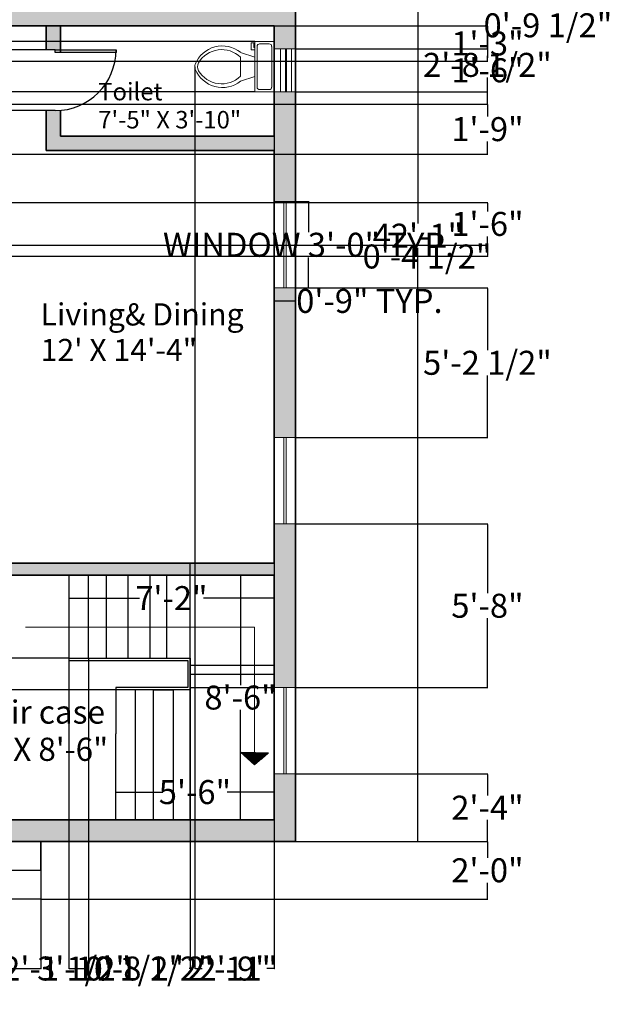
# Model space of a CAD drawing. Units: inches. Extents: x 46 to 946, y 121 to 740.
# Tile 3 of 4: x 287 to 533, y 121 to 531. Entities that reach past the tile are written whole.
import ezdxf

# ---------------------------------------------------------------- set-up
doc = ezdxf.new("R2010")
doc.units = ezdxf.units.IN
doc.header["$MEASUREMENT"] = 0
for name, color, linetype, lineweight in [('A-ANNO-DIMS', 2, 'Continuous', 18), ('A-ANNO-SYMB', 7, 'Continuous', 18), ('A-AREA-IDEN', 7, 'Continuous', 25), ('A-DOOR', 3, 'Continuous', 25), ('A-FLOR-FIXT', 9, 'Continuous', 18), ('A-FLOR-STRS', 7, 'Continuous', 25), ('A-GLAZ', 4, 'Continuous', 18), ('A-WALL', 7, 'Continuous', 35), ('A-WALL-PATT', 8, 'Continuous', 13)]:
    doc.layers.add(name, color=color, linetype=linetype, lineweight=lineweight)
doc.styles.get("Standard").update_dxf_attribs({"font": 'arial.ttf'})
doc.dimstyles.get("Standard").update_dxf_attribs({"dimtxt": 10, "dimasz": 0.18, "dimexe": 0.18, "dimexo": 0.0625, "dimgap": 0.09, "dimtad": 0, "dimtih": 1, "dimtoh": 1, "dimdec": 0, "dimzin": 0, "dimdsep": 46, "dimlunit": 3, "dimtxsty": 'Standard', "dimcen": 0.09, "dimadec": 0, "dimazin": 0, "dimtfac": 1, "dimtdec": 0, "dimtofl": 0, "dimtmove": 0, "dimatfit": 3, "dimfxl": 1, "dimtolj": 1, "dimtzin": 0, "dimarcsym": 0})

# ---------------------------------------------------------------- blocks, each defined once
blk = doc.blocks.new('*U3')
for p, q in [((0, 0), (0, -6)), ((40, 0), (40, -6))]:
    blk.add_line(p, q)
blk.add_lwpolyline([(0, 0), (0, 40), (1.75, 40), (1.75, 0)], close=True)
blk.add_arc((0, 0), 40, 0, 90)
blk = doc.blocks.new('*D7')
at = {"layer": 'A-ANNO-DIMS', "color": 0, "lineweight": -2, "transparency": 16777216}
for p, q in [((307.86, 291.97), (307.86, 289.72)), ((393.48, 291.97), (393.48, 289.72)), ((308.04, 289.9), (337.33, 289.9)), ((393.3, 289.9), (364.01, 289.9))]:
    blk.add_line(p, q, dxfattribs=at)
at = {"layer": 'A-ANNO-DIMS', "color": 0, "transparency": 16777216}
for points in [[(308.04, 289.93), (308.04, 289.87), (307.86, 289.9)], [(393.3, 289.93), (393.3, 289.87), (393.48, 289.9)]]:
    blk.add_solid(points, dxfattribs=at)
at = {"layer": 'Defpoints', "color": 0, "transparency": 16777216}
for p in [(307.86, 292.03), (393.48, 292.03), (393.48, 289.9)]:
    blk.add_point(p, dxfattribs=at)
at = {"layer": 'A-ANNO-DIMS', "color": 0, "transparency": 16777216, "insert": (350.67, 289.9), "char_height": 10, "attachment_point": 5}
blk.add_mtext('\\A1;7\'-2"', dxfattribs=at)
blk = doc.blocks.new('*D8')
at = {"layer": 'A-ANNO-DIMS', "color": 0, "lineweight": -2, "transparency": 16777216}
for p, q in [((387.34, 299.46), (379.31, 299.46)), ((379.49, 299.28), (379.49, 253.66)), ((379.49, 197.64), (379.49, 243.27)), ((387.34, 197.46), (379.31, 197.46))]:
    blk.add_line(p, q, dxfattribs=at)
at = {"layer": 'A-ANNO-DIMS', "color": 0, "transparency": 16777216}
for points in [[(379.46, 299.28), (379.52, 299.28), (379.49, 299.46)], [(379.46, 197.64), (379.52, 197.64), (379.49, 197.46)]]:
    blk.add_solid(points, dxfattribs=at)
at = {"layer": 'Defpoints', "color": 0, "transparency": 16777216}
for p in [(387.4, 299.46), (379.49, 197.46), (387.4, 197.46)]:
    blk.add_point(p, dxfattribs=at)
at = {"layer": 'A-ANNO-DIMS', "color": 0, "transparency": 16777216, "insert": (379.49, 248.46), "char_height": 10, "attachment_point": 5}
blk.add_mtext('\\A1;8\'-6"', dxfattribs=at)
blk = doc.blocks.new('*D9')
at = {"layer": 'A-ANNO-DIMS', "color": 0, "lineweight": -2, "transparency": 16777216}
for p, q in [((327.48, 197.52), (327.48, 209.23)), ((327.66, 209.05), (347.1, 209.05)), ((393.3, 209.05), (373.86, 209.05)), ((393.48, 197.52), (393.48, 209.23))]:
    blk.add_line(p, q, dxfattribs=at)
at = {"layer": 'A-ANNO-DIMS', "color": 0, "transparency": 16777216}
for points in [[(327.66, 209.08), (327.66, 209.02), (327.48, 209.05)], [(393.3, 209.08), (393.3, 209.02), (393.48, 209.05)]]:
    blk.add_solid(points, dxfattribs=at)
at = {"layer": 'Defpoints', "color": 0, "transparency": 16777216}
for p in [(393.48, 209.05), (327.48, 197.46), (393.48, 197.46)]:
    blk.add_point(p, dxfattribs=at)
at = {"layer": 'A-ANNO-DIMS', "color": 0, "transparency": 16777216, "insert": (360.48, 209.05), "char_height": 10, "attachment_point": 5}
blk.add_mtext('\\A1;5\'-6"', dxfattribs=at)
blk = doc.blocks.new('*D11')
at = {"layer": 'A-ANNO-DIMS', "color": 0, "lineweight": -2, "transparency": 16777216}
for p, q in [((402.54, 693.46), (453.64, 693.46)), ((453.46, 693.28), (453.46, 446.07)), ((453.46, 188.64), (453.46, 435.85)), ((402.54, 188.46), (453.64, 188.46))]:
    blk.add_line(p, q, dxfattribs=at)
at = {"layer": 'A-ANNO-DIMS', "color": 0, "transparency": 16777216}
for points in [[(453.43, 693.28), (453.49, 693.28), (453.46, 693.46)], [(453.43, 188.64), (453.49, 188.64), (453.46, 188.46)]]:
    blk.add_solid(points, dxfattribs=at)
at = {"layer": 'Defpoints', "color": 0, "transparency": 16777216}
for p in [(402.48, 693.46), (402.48, 188.46), (453.46, 188.46)]:
    blk.add_point(p, dxfattribs=at)
at = {"layer": 'A-ANNO-DIMS', "color": 0, "transparency": 16777216, "insert": (453.46, 440.96), "char_height": 10, "attachment_point": 5}
blk.add_mtext('\\A1;42\'-1"', dxfattribs=at)
blk = doc.blocks.new('*U13')
for p, q in [((241, -152), (241, -51)), ((-203, -216), (-203, -203)), ((-178, -203), (-178, -241)), ((-102, -203), (-152, -356)), ((102, -203), (152, -356)), ((-254, -216), (-203, -216)), ((-254, -241), (-254, -216)), ((-178, -241), (-254, -241)), ((102, -356), (-102, -356))]:
    blk.add_line(p, q)
blk.add_lwpolyline([(267, -203), (267, 0), (-267, 0), (-267, -203)], close=True)
for points in [[(-241, -51), (-241, -152)], [(216, -25), (-216, -25)], [(-216, -178), (216, -178)]]:
    blk.add_lwpolyline(points)
for centre, radius, start, end in [((-219, -48), 22.5, 81.8699, 188.1301), ((219, -48), 22.5, 351.8699, 98.1301), ((-219, -156), 22.5, 171.8699, 278.1301), ((219, -156), 22.5, 261.8699, 8.1301), ((89, -548), 309, 141.4691, 247.9714), ((107, -554), 288, 136.3677, 238.9468), ((-89, -548), 309, 292.0284, 38.5307), ((-107, -554), 288, 301.053, 43.6321), ((0, -708), 102, 245.7318, 294.2682), ((0, -737), 102, 254.8605, 285.1395)]:
    blk.add_arc(centre, radius, start, end)
blk = doc.blocks.new('WIN-36IN')
for p, q in [((9, 36), (0, 36)), ((0, 0), (0, 36)), ((4, 36), (4, 0)), ((5, 36), (5, 0)), ((9, 36), (9, 0)), ((9, 0), (0, 0)), ((9, 0), (0, 0))]:
    blk.add_line(p, q)
blk = doc.blocks.new('ARROW-DIRECTION')
h = blk.add_hatch()
h.set_pattern_fill('ANSI31', color=256, angle=180)
h.set_pattern_definition([(225, (391.19844, 225.63338), (0.088388348, -0.088388348), [])])
h.paths.add_polyline_path([(0, 0.27), (11.71, 0), (5.84, 5.18)])
for p, q in [((5.84, 5.18), (0, 0.27)), ((5.84, 5.18), (11.71, 0)), ((11.71, 0), (5.84, 5.18))]:
    blk.add_line(p, q)
blk = doc.blocks.new('*D20')
at = {"layer": 'A-ANNO-DIMS', "color": 0, "lineweight": -2, "transparency": 16777216}
for p, q in [((402.54, 455.17), (408.06, 455.17)), ((407.88, 454.99), (407.88, 442.43)), ((407.88, 419.35), (407.88, 431.9)), ((402.54, 419.17), (408.06, 419.17))]:
    blk.add_line(p, q, dxfattribs=at)
at = {"layer": 'A-ANNO-DIMS', "color": 0, "transparency": 16777216}
for points in [[(407.85, 454.99), (407.91, 454.99), (407.88, 455.17)], [(407.85, 419.35), (407.91, 419.35), (407.88, 419.17)]]:
    blk.add_solid(points, dxfattribs=at)
at = {"layer": 'Defpoints', "color": 0, "transparency": 16777216}
for p in [(402.48, 455.17), (407.88, 455.17), (402.48, 419.17)]:
    blk.add_point(p, dxfattribs=at)
at = {"layer": 'A-ANNO-DIMS', "color": 0, "transparency": 16777216, "insert": (407.88, 437.17), "char_height": 10, "attachment_point": 5}
blk.add_mtext('\\A1;WINDOW 3\'-0" TYP.', dxfattribs=at)
blk = doc.blocks.new('*D21')
at = {"layer": 'A-ANNO-DIMS', "color": 0, "lineweight": -2, "transparency": 16777216}
for p, q in [((393.48, 419.1), (393.48, 413.59)), ((402.48, 419.1), (402.48, 413.59)), ((393.66, 413.77), (402.3, 413.77)), ((402.48, 413.77), (402.66, 413.77))]:
    blk.add_line(p, q, dxfattribs=at)
at = {"layer": 'A-ANNO-DIMS', "color": 0, "transparency": 16777216}
for points in [[(393.66, 413.8), (393.66, 413.74), (393.48, 413.77)], [(402.3, 413.8), (402.3, 413.74), (402.48, 413.77)]]:
    blk.add_solid(points, dxfattribs=at)
at = {"layer": 'Defpoints', "color": 0, "transparency": 16777216}
for p in [(393.48, 419.17), (402.48, 419.17), (402.48, 413.77)]:
    blk.add_point(p, dxfattribs=at)
at = {"layer": 'A-ANNO-DIMS', "color": 0, "transparency": 16777216, "insert": (433.22, 413.77), "char_height": 10, "attachment_point": 5}
blk.add_mtext('\\A1;0\'-9" TYP.', dxfattribs=at)
blk = doc.blocks.new('*D25')
at = {"layer": 'A-ANNO-DIMS', "color": 0, "lineweight": -2, "transparency": 16777216}
for p, q in [((249.48, 164.4), (249.48, 135.33)), ((296.21, 164.4), (296.21, 135.33)), ((249.66, 135.51), (296.03, 135.51)), ((296.21, 135.51), (296.39, 135.51))]:
    blk.add_line(p, q, dxfattribs=at)
at = {"layer": 'A-ANNO-DIMS', "color": 0, "transparency": 16777216}
for points in [[(249.66, 135.54), (249.66, 135.48), (249.48, 135.51)], [(296.03, 135.54), (296.03, 135.48), (296.21, 135.51)]]:
    blk.add_solid(points, dxfattribs=at)
at = {"layer": 'Defpoints', "color": 0, "transparency": 16777216}
for p in [(249.48, 164.46), (296.21, 164.46), (296.21, 135.51)]:
    blk.add_point(p, dxfattribs=at)
at = {"layer": 'A-ANNO-DIMS', "color": 0, "transparency": 16777216, "insert": (325.3, 135.51), "char_height": 10, "attachment_point": 5}
blk.add_mtext('\\A1;3\'-10 1/2"', dxfattribs=at)
blk = doc.blocks.new('*D26')
at = {"layer": 'A-ANNO-DIMS', "color": 0, "lineweight": -2, "transparency": 16777216}
for p, q in [((296.27, 188.46), (482.61, 188.46)), ((482.43, 188.28), (482.43, 181.66)), ((482.43, 164.64), (482.43, 171.27)), ((296.27, 164.46), (482.61, 164.46))]:
    blk.add_line(p, q, dxfattribs=at)
at = {"layer": 'A-ANNO-DIMS', "color": 0, "transparency": 16777216}
for points in [[(482.4, 188.28), (482.46, 188.28), (482.43, 188.46)], [(482.4, 164.64), (482.46, 164.64), (482.43, 164.46)]]:
    blk.add_solid(points, dxfattribs=at)
at = {"layer": 'Defpoints', "color": 0, "transparency": 16777216}
for p in [(296.21, 188.46), (482.43, 188.46), (296.21, 164.46)]:
    blk.add_point(p, dxfattribs=at)
at = {"layer": 'A-ANNO-DIMS', "color": 0, "transparency": 16777216, "insert": (482.43, 176.46), "char_height": 10, "attachment_point": 5}
blk.add_mtext('\\A1;2\'-0"', dxfattribs=at)
blk = doc.blocks.new('*D37')
at = {"layer": 'A-ANNO-DIMS', "color": 0, "lineweight": -2, "transparency": 16777216}
for p, q in [((402.54, 216.63), (482.61, 216.63)), ((482.43, 216.45), (482.43, 207.66)), ((482.43, 188.64), (482.43, 197.44)), ((402.54, 188.46), (482.61, 188.46))]:
    blk.add_line(p, q, dxfattribs=at)
at = {"layer": 'A-ANNO-DIMS', "color": 0, "transparency": 16777216}
for points in [[(482.4, 216.45), (482.46, 216.45), (482.43, 216.63)], [(482.4, 188.64), (482.46, 188.64), (482.43, 188.46)]]:
    blk.add_solid(points, dxfattribs=at)
at = {"layer": 'Defpoints', "color": 0, "transparency": 16777216}
for p in [(402.48, 216.63), (482.43, 216.63), (402.48, 188.46)]:
    blk.add_point(p, dxfattribs=at)
at = {"layer": 'A-ANNO-DIMS', "color": 0, "transparency": 16777216, "insert": (482.43, 202.55), "char_height": 10, "attachment_point": 5}
blk.add_mtext('\\A1;2\'-4"', dxfattribs=at)
blk = doc.blocks.new('*D38')
at = {"layer": 'A-ANNO-DIMS', "color": 0, "lineweight": -2, "transparency": 16777216}
for p, q in [((402.54, 320.8), (482.61, 320.8)), ((482.43, 320.62), (482.43, 291.91)), ((482.43, 252.81), (482.43, 281.52)), ((402.54, 252.63), (482.61, 252.63))]:
    blk.add_line(p, q, dxfattribs=at)
at = {"layer": 'A-ANNO-DIMS', "color": 0, "transparency": 16777216}
for points in [[(482.4, 320.62), (482.46, 320.62), (482.43, 320.8)], [(482.4, 252.81), (482.46, 252.81), (482.43, 252.63)]]:
    blk.add_solid(points, dxfattribs=at)
at = {"layer": 'Defpoints', "color": 0, "transparency": 16777216}
for p in [(402.48, 320.8), (482.43, 320.8), (402.48, 252.63)]:
    blk.add_point(p, dxfattribs=at)
at = {"layer": 'A-ANNO-DIMS', "color": 0, "transparency": 16777216, "insert": (482.43, 286.72), "char_height": 10, "attachment_point": 5}
blk.add_mtext('\\A1;5\'-8"', dxfattribs=at)
blk = doc.blocks.new('*D39')
at = {"layer": 'A-ANNO-DIMS', "color": 0, "lineweight": -2, "transparency": 16777216}
for p, q in [((402.54, 419.17), (482.61, 419.17)), ((482.43, 418.99), (482.43, 393.25)), ((482.43, 356.98), (482.43, 382.72)), ((402.54, 356.8), (482.61, 356.8))]:
    blk.add_line(p, q, dxfattribs=at)
at = {"layer": 'A-ANNO-DIMS', "color": 0, "transparency": 16777216}
for points in [[(482.4, 418.99), (482.46, 418.99), (482.43, 419.17)], [(482.4, 356.98), (482.46, 356.98), (482.43, 356.8)]]:
    blk.add_solid(points, dxfattribs=at)
at = {"layer": 'Defpoints', "color": 0, "transparency": 16777216}
for p in [(402.48, 419.17), (482.43, 419.17), (402.48, 356.8)]:
    blk.add_point(p, dxfattribs=at)
at = {"layer": 'A-ANNO-DIMS', "color": 0, "transparency": 16777216, "insert": (482.43, 387.98), "char_height": 10, "attachment_point": 5}
blk.add_mtext('\\A1;5\'-2 1/2"', dxfattribs=at)
blk = doc.blocks.new('*D40')
at = {"layer": 'A-ANNO-DIMS', "color": 0, "lineweight": -2, "transparency": 16777216}
for p, q in [((393.54, 528.46), (482.61, 528.46)), ((482.43, 528.46), (482.43, 528.64)), ((482.43, 528.64), (482.61, 528.64)), ((482.43, 519.05), (482.43, 528.28)), ((402.54, 518.87), (482.61, 518.87))]:
    blk.add_line(p, q, dxfattribs=at)
at = {"layer": 'A-ANNO-DIMS', "color": 0, "transparency": 16777216}
for points in [[(482.4, 528.28), (482.46, 528.28), (482.43, 528.46)], [(482.4, 519.05), (482.46, 519.05), (482.43, 518.87)]]:
    blk.add_solid(points, dxfattribs=at)
at = {"layer": 'Defpoints', "color": 0, "transparency": 16777216}
for p in [(393.48, 528.46), (482.43, 528.46), (402.48, 518.87)]:
    blk.add_point(p, dxfattribs=at)
at = {"layer": 'A-ANNO-DIMS', "color": 0, "transparency": 16777216, "insert": (507.64, 528.64), "char_height": 10, "attachment_point": 5}
blk.add_mtext('\\A1;0\'-9 1/2"', dxfattribs=at)
blk = doc.blocks.new('*D41')
at = {"layer": 'A-ANNO-DIMS', "color": 0, "lineweight": -2, "transparency": 16777216}
for p, q in [((402.54, 518.87), (482.61, 518.87)), ((482.43, 518.69), (482.43, 515.07)), ((402.54, 500.87), (482.61, 500.87)), ((482.43, 501.05), (482.43, 504.68))]:
    blk.add_line(p, q, dxfattribs=at)
at = {"layer": 'A-ANNO-DIMS', "color": 0, "transparency": 16777216}
for points in [[(482.4, 518.69), (482.46, 518.69), (482.43, 518.87)], [(482.4, 501.05), (482.46, 501.05), (482.43, 500.87)]]:
    blk.add_solid(points, dxfattribs=at)
at = {"layer": 'Defpoints', "color": 0, "transparency": 16777216}
for p in [(402.48, 518.87), (482.43, 518.87), (402.48, 500.87)]:
    blk.add_point(p, dxfattribs=at)
at = {"layer": 'A-ANNO-DIMS', "color": 0, "transparency": 16777216, "insert": (482.43, 509.87), "char_height": 10, "attachment_point": 5}
blk.add_mtext('\\A1;1\'-6"', dxfattribs=at)
blk = doc.blocks.new('*D44')
at = {"layer": 'A-ANNO-DIMS', "color": 0, "lineweight": -2, "transparency": 16777216}
for p, q in [((256.37, 188.4), (256.37, 135.33)), ((281.69, 188.4), (281.69, 135.33)), ((256.55, 135.51), (281.51, 135.51)), ((281.69, 135.51), (281.87, 135.51))]:
    blk.add_line(p, q, dxfattribs=at)
at = {"layer": 'A-ANNO-DIMS', "color": 0, "transparency": 16777216}
for points in [[(256.55, 135.54), (256.55, 135.48), (256.37, 135.51)], [(281.51, 135.54), (281.51, 135.48), (281.69, 135.51)]]:
    blk.add_solid(points, dxfattribs=at)
at = {"layer": 'Defpoints', "color": 0, "transparency": 16777216}
for p in [(256.37, 188.46), (281.69, 188.46), (281.69, 135.51)]:
    blk.add_point(p, dxfattribs=at)
at = {"layer": 'A-ANNO-DIMS', "color": 0, "transparency": 16777216, "insert": (306.99, 135.51), "char_height": 10, "attachment_point": 5}
blk.add_mtext('\\A1;2\'-1 1/2"', dxfattribs=at)
blk = doc.blocks.new('*D48')
at = {"layer": 'A-ANNO-DIMS', "color": 0, "lineweight": -2, "transparency": 16777216}
for p, q in [((188.89, 454.75), (482.61, 454.75)), ((482.43, 454.57), (482.43, 451.05)), ((482.43, 437.15), (482.43, 440.66)), ((188.89, 436.97), (482.61, 436.97))]:
    blk.add_line(p, q, dxfattribs=at)
at = {"layer": 'A-ANNO-DIMS', "color": 0, "transparency": 16777216}
for points in [[(482.4, 454.57), (482.46, 454.57), (482.43, 454.75)], [(482.4, 437.15), (482.46, 437.15), (482.43, 436.97)]]:
    blk.add_solid(points, dxfattribs=at)
at = {"layer": 'Defpoints', "color": 0, "transparency": 16777216}
for p in [(188.83, 454.75), (482.43, 454.75), (188.83, 436.97)]:
    blk.add_point(p, dxfattribs=at)
at = {"layer": 'A-ANNO-DIMS', "color": 0, "transparency": 16777216, "insert": (482.43, 445.86), "char_height": 10, "attachment_point": 5}
blk.add_mtext('\\A1;1\'-6"', dxfattribs=at)
blk = doc.blocks.new('*D50')
at = {"layer": 'A-ANNO-DIMS', "color": 0, "lineweight": -2, "transparency": 16777216}
for p, q in [((195.54, 495.84), (482.61, 495.84)), ((482.43, 495.66), (482.43, 490.57)), ((482.43, 475.08), (482.43, 480.18)), ((195.54, 474.9), (482.61, 474.9))]:
    blk.add_line(p, q, dxfattribs=at)
at = {"layer": 'A-ANNO-DIMS', "color": 0, "transparency": 16777216}
for points in [[(482.4, 495.66), (482.46, 495.66), (482.43, 495.84)], [(482.4, 475.08), (482.46, 475.08), (482.43, 474.9)]]:
    blk.add_solid(points, dxfattribs=at)
at = {"layer": 'Defpoints', "color": 0, "transparency": 16777216}
for p in [(195.48, 495.84), (482.43, 495.84), (195.48, 474.9)]:
    blk.add_point(p, dxfattribs=at)
at = {"layer": 'A-ANNO-DIMS', "color": 0, "transparency": 16777216, "insert": (482.43, 485.37), "char_height": 10, "attachment_point": 5}
blk.add_mtext('\\A1;1\'-9"', dxfattribs=at)
blk = doc.blocks.new('*D55')
at = {"layer": 'A-ANNO-DIMS', "color": 0, "lineweight": -2, "transparency": 16777216}
for p, q in [((307.8, 299.46), (85.35, 299.46)), ((85.53, 299.28), (85.53, 287.43)), ((85.53, 265.06), (85.53, 276.91)), ((307.8, 264.88), (85.35, 264.88))]:
    blk.add_line(p, q, dxfattribs=at)
at = {"layer": 'A-ANNO-DIMS', "color": 0, "transparency": 16777216}
for points in [[(85.5, 299.28), (85.56, 299.28), (85.53, 299.46)], [(85.5, 265.06), (85.56, 265.06), (85.53, 264.88)]]:
    blk.add_solid(points, dxfattribs=at)
at = {"layer": 'Defpoints', "color": 0, "transparency": 16777216}
for p in [(307.86, 299.46), (85.53, 264.88), (307.86, 264.88)]:
    blk.add_point(p, dxfattribs=at)
at = {"layer": 'A-ANNO-DIMS', "color": 0, "transparency": 16777216, "insert": (85.53, 282.17), "char_height": 10, "attachment_point": 5}
blk.add_mtext('\\A1;2\'-10 1/2"', dxfattribs=at)
blk = doc.blocks.new('*D56')
at = {"layer": 'A-ANNO-DIMS', "color": 0, "lineweight": -2, "transparency": 16777216}
for p, q in [((307.86, 264.81), (307.86, 135.33)), ((316.14, 264.81), (316.14, 135.33)), ((308.04, 135.51), (315.96, 135.51)), ((316.14, 135.51), (316.32, 135.51))]:
    blk.add_line(p, q, dxfattribs=at)
at = {"layer": 'A-ANNO-DIMS', "color": 0, "transparency": 16777216}
for points in [[(308.04, 135.54), (308.04, 135.48), (307.86, 135.51)], [(315.96, 135.54), (315.96, 135.48), (316.14, 135.51)]]:
    blk.add_solid(points, dxfattribs=at)
at = {"layer": 'Defpoints', "color": 0, "transparency": 16777216}
for p in [(307.86, 264.88), (316.14, 264.88), (316.14, 135.51)]:
    blk.add_point(p, dxfattribs=at)
at = {"layer": 'A-ANNO-DIMS', "color": 0, "transparency": 16777216, "insert": (341.35, 135.51), "char_height": 10, "attachment_point": 5}
blk.add_mtext('\\A1;0\'-8 1/2"', dxfattribs=at)
blk = doc.blocks.new('*D57')
at = {"layer": 'A-ANNO-DIMS', "color": 0, "lineweight": -2, "transparency": 16777216}
for p, q in [((327.41, 251.63), (85.35, 251.63)), ((85.53, 251.45), (85.53, 229.74)), ((85.53, 197.64), (85.53, 219.35)), ((327.41, 197.46), (85.35, 197.46))]:
    blk.add_line(p, q, dxfattribs=at)
at = {"layer": 'A-ANNO-DIMS', "color": 0, "transparency": 16777216}
for points in [[(85.5, 251.45), (85.56, 251.45), (85.53, 251.63)], [(85.5, 197.64), (85.56, 197.64), (85.53, 197.46)]]:
    blk.add_solid(points, dxfattribs=at)
at = {"layer": 'Defpoints', "color": 0, "transparency": 16777216}
for p in [(327.48, 251.63), (85.53, 197.46), (327.48, 197.46)]:
    blk.add_point(p, dxfattribs=at)
at = {"layer": 'A-ANNO-DIMS', "color": 0, "transparency": 16777216, "insert": (85.53, 224.55), "char_height": 10, "attachment_point": 5}
blk.add_mtext('\\A1;4\'-6"', dxfattribs=at)
blk = doc.blocks.new('*D58')
at = {"layer": 'A-ANNO-DIMS', "color": 0, "lineweight": -2, "transparency": 16777216}
for p, q in [((358.476776, 251.569905), (358.476776, 135.331347)), ((393.476776, 252.569905), (393.476776, 135.331347)), ((358.296776, 135.511347), (358.116776, 135.511347)), ((393.656776, 135.511347), (393.836776, 135.511347))]:
    blk.add_line(p, q, dxfattribs=at)
at = {"layer": 'A-ANNO-DIMS', "color": 0, "transparency": 16777216}
for points in [[(358.296776, 135.541347), (358.296776, 135.481347), (358.476776, 135.511347)], [(393.656776, 135.541347), (393.656776, 135.481347), (393.476776, 135.511347)]]:
    blk.add_solid(points, dxfattribs=at)
at = {"layer": 'Defpoints', "color": 0, "transparency": 16777216}
for p in [(358.476776, 251.632405), (393.476776, 252.632405), (393.476776, 135.511347)]:
    blk.add_point(p, dxfattribs=at)
at = {"layer": 'A-ANNO-DIMS', "color": 0, "transparency": 16777216, "insert": (375.976776, 135.511347), "char_height": 10, "attachment_point": 5}
blk.add_mtext('\\A1;2\'-11"', dxfattribs=at)
blk = doc.blocks.new('*D59')
at = {"layer": 'A-ANNO-DIMS', "color": 0, "lineweight": -2, "transparency": 16777216}
for p, q in [((360.48, 511.31), (360.48, 135.33)), ((393.48, 500.81), (393.48, 135.33)), ((360.66, 135.51), (363.51, 135.51)), ((393.3, 135.51), (390.44, 135.51))]:
    blk.add_line(p, q, dxfattribs=at)
at = {"layer": 'A-ANNO-DIMS', "color": 0, "transparency": 16777216}
for points in [[(360.66, 135.54), (360.66, 135.48), (360.48, 135.51)], [(393.3, 135.54), (393.3, 135.48), (393.48, 135.51)]]:
    blk.add_solid(points, dxfattribs=at)
at = {"layer": 'Defpoints', "color": 0, "transparency": 16777216}
for p in [(360.48, 511.37), (393.48, 500.87), (393.48, 135.51)]:
    blk.add_point(p, dxfattribs=at)
at = {"layer": 'A-ANNO-DIMS', "color": 0, "transparency": 16777216, "insert": (376.98, 135.51), "char_height": 10, "attachment_point": 5}
blk.add_mtext('\\A1;2\'-9"', dxfattribs=at)
blk = doc.blocks.new('*D60')
at = {"layer": 'A-ANNO-DIMS', "color": 0, "lineweight": -2, "transparency": 16777216}
for p, q in [((385.41, 521.87), (85.35, 521.87)), ((85.53, 521.69), (85.53, 516.57)), ((85.53, 501.05), (85.53, 506.18)), ((385.41, 500.87), (85.35, 500.87))]:
    blk.add_line(p, q, dxfattribs=at)
at = {"layer": 'A-ANNO-DIMS', "color": 0, "transparency": 16777216}
for points in [[(85.5, 521.69), (85.56, 521.69), (85.53, 521.87)], [(85.5, 501.05), (85.56, 501.05), (85.53, 500.87)]]:
    blk.add_solid(points, dxfattribs=at)
at = {"layer": 'Defpoints', "color": 0, "transparency": 16777216}
for p in [(85.53, 521.87), (385.48, 521.87), (385.48, 500.87)]:
    blk.add_point(p, dxfattribs=at)
at = {"layer": 'A-ANNO-DIMS', "color": 0, "transparency": 16777216, "insert": (85.53, 511.37), "char_height": 10, "attachment_point": 5}
blk.add_mtext('\\A1;1\'-9"', dxfattribs=at)
blk = doc.blocks.new('*D61')
at = {"layer": 'A-ANNO-DIMS', "color": 0, "lineweight": -2, "transparency": 16777216}
for p, q in [((304.41, 528.46), (85.35, 528.46)), ((85.53, 528.28), (85.53, 518.59)), ((298.41, 518.41), (85.35, 518.41)), ((85.53, 518.23), (85.35, 518.23)), ((85.53, 518.41), (85.53, 518.23))]:
    blk.add_line(p, q, dxfattribs=at)
at = {"layer": 'A-ANNO-DIMS', "color": 0, "transparency": 16777216}
for points in [[(85.5, 528.28), (85.56, 528.28), (85.53, 528.46)], [(85.5, 518.59), (85.56, 518.59), (85.53, 518.41)]]:
    blk.add_solid(points, dxfattribs=at)
at = {"layer": 'Defpoints', "color": 0, "transparency": 16777216}
for p in [(304.48, 528.46), (85.53, 518.41), (298.48, 518.41)]:
    blk.add_point(p, dxfattribs=at)
at = {"layer": 'A-ANNO-DIMS', "color": 0, "transparency": 16777216, "insert": (68.08, 518.23), "char_height": 10, "attachment_point": 5}
blk.add_mtext('\\A1;0\'-10"', dxfattribs=at)
blk = doc.blocks.new('*D62')
at = {"layer": 'A-ANNO-DIMS', "color": 0, "lineweight": -2, "transparency": 16777216}
for p, q in [((298.41, 518.41), (85.35, 518.41)), ((85.53, 518.23), (85.53, 511.01)), ((85.53, 493.27), (85.53, 500.49)), ((298.41, 493.09), (85.35, 493.09))]:
    blk.add_line(p, q, dxfattribs=at)
at = {"layer": 'A-ANNO-DIMS', "color": 0, "transparency": 16777216}
for points in [[(85.5, 518.23), (85.56, 518.23), (85.53, 518.41)], [(85.5, 493.27), (85.56, 493.27), (85.53, 493.09)]]:
    blk.add_solid(points, dxfattribs=at)
at = {"layer": 'Defpoints', "color": 0, "transparency": 16777216}
for p in [(298.48, 518.41), (85.53, 493.09), (298.48, 493.09)]:
    blk.add_point(p, dxfattribs=at)
at = {"layer": 'A-ANNO-DIMS', "color": 0, "transparency": 16777216, "insert": (85.53, 505.75), "char_height": 10, "attachment_point": 5}
blk.add_mtext('\\A1;2\'-1 1/2"', dxfattribs=at)
blk = doc.blocks.new('*D63')
at = {"layer": 'A-ANNO-DIMS', "color": 0, "lineweight": -2, "transparency": 16777216}
for p, q in [((195.54, 528.46), (482.61, 528.46)), ((482.43, 528.28), (482.43, 517.41)), ((482.43, 496.02), (482.43, 506.89)), ((195.54, 495.84), (482.61, 495.84))]:
    blk.add_line(p, q, dxfattribs=at)
at = {"layer": 'A-ANNO-DIMS', "color": 0, "transparency": 16777216}
for points in [[(482.4, 528.28), (482.46, 528.28), (482.43, 528.46)], [(482.4, 496.02), (482.46, 496.02), (482.43, 495.84)]]:
    blk.add_solid(points, dxfattribs=at)
at = {"layer": 'Defpoints', "color": 0, "transparency": 16777216}
for p in [(195.48, 528.46), (195.48, 495.84), (482.43, 495.84)]:
    blk.add_point(p, dxfattribs=at)
at = {"layer": 'A-ANNO-DIMS', "color": 0, "transparency": 16777216, "insert": (482.43, 512.15), "char_height": 10, "attachment_point": 5}
blk.add_mtext('\\A1;2\'-8 1/2"', dxfattribs=at)
blk = doc.blocks.new('*D67')
at = {"layer": 'A-ANNO-DIMS', "color": 0, "lineweight": -2, "transparency": 16777216}
for p, q in [((159.54, 528.46), (482.61, 528.46)), ((482.43, 528.28), (482.43, 526.27)), ((150.66, 513.68), (482.61, 513.68)), ((482.43, 513.86), (482.43, 515.87))]:
    blk.add_line(p, q, dxfattribs=at)
at = {"layer": 'A-ANNO-DIMS', "color": 0, "transparency": 16777216}
for points in [[(482.4, 528.28), (482.46, 528.28), (482.43, 528.46)], [(482.4, 513.86), (482.46, 513.86), (482.43, 513.68)]]:
    blk.add_solid(points, dxfattribs=at)
at = {"layer": 'Defpoints', "color": 0, "transparency": 16777216}
for p in [(159.48, 528.46), (482.43, 528.46), (150.6, 513.68)]:
    blk.add_point(p, dxfattribs=at)
at = {"layer": 'A-ANNO-DIMS', "color": 0, "transparency": 16777216, "insert": (482.43, 521.07), "char_height": 10, "attachment_point": 5}
blk.add_mtext('\\A1;1\'-3"', dxfattribs=at)
blk = doc.blocks.new('*D69')
at = {"layer": 'A-ANNO-DIMS', "color": 0, "lineweight": -2, "transparency": 16777216}
for p, q in [((188.89, 436.97), (482.61, 436.97)), ((482.43, 436.79), (482.43, 432.64)), ((195.54, 432.46), (482.61, 432.46)), ((482.43, 432.28), (482.25, 432.28)), ((482.43, 432.46), (482.43, 432.28))]:
    blk.add_line(p, q, dxfattribs=at)
at = {"layer": 'A-ANNO-DIMS', "color": 0, "transparency": 16777216}
for points in [[(482.4, 436.79), (482.46, 436.79), (482.43, 436.97)], [(482.4, 432.64), (482.46, 432.64), (482.43, 432.46)]]:
    blk.add_solid(points, dxfattribs=at)
at = {"layer": 'Defpoints', "color": 0, "transparency": 16777216}
for p in [(188.83, 436.97), (195.48, 432.46), (482.43, 432.46)]:
    blk.add_point(p, dxfattribs=at)
at = {"layer": 'A-ANNO-DIMS', "color": 0, "transparency": 16777216, "insert": (457.21, 432.28), "char_height": 10, "attachment_point": 5}
blk.add_mtext('\\A1;0\'-4 1/2"', dxfattribs=at)

msp = doc.modelspace()

# ---------------------------------------------------------------- hatches: boundary and pattern name
at = {"layer": 'A-WALL-PATT'}
h = msp.add_hatch(color=256, dxfattribs=at)
h.dxf.hatch_style = 1
h.paths.add_polyline_path([(256.37, 197.46), (249.48, 197.46), (249.48, 258.28), (245.68, 258.28, -0.021769), (243.48, 258.37), (243.48, 197.46), (221.61, 197.46), (221.61, 188.46), (243.48, 188.46), (256.37, 188.46), (256.37, 192.26)])
h.paths.add_polyline_path([(164.78, 197.46), (123.48, 197.46), (123.48, 224.01), (114.48, 224.01), (114.48, 188.46), (164.78, 188.46)])
h.paths.add_polyline_path([(402.48, 216.63), (393.48, 216.63), (393.48, 197.46), (327.48, 197.46), (281.15, 197.46, -0.051771), (281.69, 192.26), (281.69, 188.46), (402.48, 188.46)])
h.paths.add_polyline_path([(123.48, 346.49), (114.48, 346.49), (114.48, 280.83), (123.48, 280.83), (123.48, 299.46), (243.48, 299.46), (243.48, 283.6), (245.68, 283.6), (249.48, 283.6), (249.48, 299.46), (256.37, 299.46), (256.37, 303.26), (256.37, 304.46), (249.48, 304.46), (249.48, 432.46), (243.48, 432.46), (232.61, 432.46), (232.61, 426.46), (243.48, 426.46), (243.48, 305.46), (123.48, 305.46)])
h.paths.add_polyline_path([(231.5, 428.66), (232.61, 428.66), (232.61, 403.34), (231.5, 403.34), (231.5, 403.37, -0.376395), (207.38, 426.46), (123.48, 426.46), (123.48, 403.31), (114.48, 403.31), (114.48, 453.42), (123.48, 453.42), (123.48, 432.46), (195.48, 432.46), (195.48, 474.9), (201.48, 474.9), (201.48, 432.46), (207.29, 432.46), (207.29, 428.66, 0.401453), (231.5, 403.37)])
h.paths.add_polyline_path([(211.14, 534.46), (123.48, 534.46), (123.48, 573.18), (114.48, 573.18), (114.48, 510.24), (123.48, 510.24), (123.48, 528.46), (195.48, 528.46), (195.48, 495.84), (201.48, 495.84), (201.48, 528.46), (211.04, 528.46), (211.04, 532.26, -0.021769)])
h.paths.add_polyline_path([(123.48, 684.46), (243.48, 684.46), (243.48, 534.46), (236.36, 534.46), (236.36, 532.26), (236.36, 528.46), (256.37, 528.46), (256.37, 532.26), (256.37, 534.46), (249.48, 534.46), (249.48, 684.46), (393.48, 684.46), (393.48, 647.42), (402.48, 647.42), (402.48, 693.46), (114.48, 693.46), (114.48, 630), (123.48, 630)])
h.paths.add_polyline_path([(402.48, 590.59), (393.48, 590.59), (393.48, 534.46), (281.59, 534.46, -0.021769), (281.69, 532.26), (281.69, 528.46), (298.48, 528.46), (298.48, 518.41), (302.28, 518.41), (304.48, 518.41), (304.48, 528.46), (393.48, 528.46), (393.48, 518.87), (402.48, 518.87)])
h.paths.add_polyline_path([(402.48, 500.87), (393.48, 500.87), (393.48, 482.46), (304.48, 482.46), (304.48, 493.19, -0.021769), (302.28, 493.09), (298.48, 493.09), (298.48, 482.46), (298.48, 476.46), (304.48, 476.46), (393.48, 476.46), (393.48, 455.17), (402.48, 455.17)])
h.paths.add_polyline_path([(402.48, 419.17), (393.48, 419.17), (393.48, 356.8), (402.48, 356.8)])
h.paths.add_polyline_path([(358.48, 304.46), (281.66, 304.46, -0.01187), (281.69, 303.26), (281.69, 299.46), (358.48, 299.46)])
h = msp.add_hatch(color=256, dxfattribs=at)
h.dxf.hatch_style = 1
h.paths.add_polyline_path([(402.48, 320.8), (393.48, 320.8), (393.48, 304.46), (358.48, 304.46), (358.48, 299.46), (393.48, 299.46), (393.48, 298.46), (393.48, 252.63), (402.48, 252.63)])

# ---------------------------------------------------------------- linework, layer by layer
at = {"layer": 'A-ANNO-SYMB'}
for p, q in [((289.86, 277.81), (385.35, 277.81)), ((385.35, 277.81), (385.35, 225.5)), ((391.2, 225.37), (379.49, 225.63))]:
    msp.add_line(p, q, dxfattribs=at)
at = {"layer": 'A-FLOR-STRS'}
for p, q in [((358.48, 264.88), (358.48, 304.46)), ((393.48, 299.46), (307.86, 299.46)), ((307.86, 299.46), (307.86, 263.88)), ((316.14, 264.88), (316.14, 299.46)), ((316.14, 299.46), (323.45, 299.46)), ((323.45, 299.46), (323.45, 264.88)), ((332.67, 264.88), (332.67, 299.46)), ((332.67, 299.46), (341.73, 299.46)), ((341.73, 299.46), (341.73, 264.88)), ((348.82, 264.88), (348.82, 299.46)), ((307.86, 264.88), (357.48, 264.88)), ((307.86, 263.88), (357.48, 263.88)), ((323.45, 264.88), (332.67, 264.88)), ((341.73, 264.88), (348.82, 264.88)), ((357.48, 264.88), (358.48, 264.88)), ((357.48, 263.88), (357.48, 252.63)), ((358.48, 264.88), (358.48, 263.88)), ((358.48, 197.46), (358.48, 264.88)), ((358.48, 263.88), (358.48, 252.63)), ((358.48, 263.88), (358.48, 252.63)), ((358.48, 261.92), (393.48, 261.92)), ((358.48, 258.25), (393.48, 258.25)), ((357.48, 252.63), (327.48, 252.63)), ((327.48, 252.63), (327.48, 233.33)), ((357.48, 251.63), (327.48, 251.63)), ((335.63, 251.63), (335.63, 197.46)), ((343.27, 197.46), (343.27, 251.63)), ((343.27, 251.63), (351.46, 251.63)), ((351.46, 251.63), (351.46, 197.46)), ((358.48, 251.63), (357.48, 251.63)), ((358.48, 252.63), (358.48, 251.63)), ((358.48, 252.63), (393.48, 252.63)), ((358.48, 252.13), (358.48, 197.46)), ((327.48, 197.46), (327.48, 233.33)), ((393.48, 197.46), (327.48, 197.46)), ((335.63, 197.46), (343.27, 197.46)), ((351.46, 197.46), (366.1, 197.46)), ((296.21, 176.46), (296.21, 188.46)), ((296.21, 188.46), (296.21, 164.46)), ((249.48, 176.46), (296.21, 176.46)), ((296.21, 164.46), (249.48, 164.46))]:
    msp.add_line(p, q, dxfattribs=at)
at = {"layer": 'A-GLAZ'}
for p, q in [((402.48, 518.87), (393.48, 518.87)), ((396.21, 500.87), (396.21, 518.87)), ((398.21, 518.87), (398.21, 500.87)), ((398.71, 518.87), (398.71, 500.87)), ((400.71, 518.87), (400.71, 500.87)), ((402.48, 500.87), (393.48, 500.87)), ((400.71, 500.87), (396.21, 500.87))]:
    msp.add_line(p, q, dxfattribs=at)
at = {"layer": 'A-WALL'}
for p, q in [((402.48, 693.46), (402.48, 188.46)), ((281.69, 528.46), (298.48, 528.46)), ((298.48, 518.41), (298.48, 528.46)), ((304.48, 528.46), (393.48, 528.46)), ((304.48, 517.31), (304.48, 528.46)), ((393.48, 528.46), (393.48, 482.46)), ((393.48, 528.46), (393.48, 482.46)), ((298.48, 482.46), (298.48, 493.09)), ((304.48, 482.46), (304.48, 493.19)), ((298.48, 482.46), (298.48, 476.46)), ((393.48, 482.46), (304.48, 482.46)), ((298.48, 476.46), (304.48, 476.46)), ((393.48, 476.46), (304.48, 476.46)), ((393.48, 476.46), (393.48, 304.46)), ((393.48, 304.46), (281.66, 304.46)), ((281.69, 299.46), (393.48, 299.46)), ((393.48, 299.46), (393.48, 299.46)), ((393.48, 298.46), (393.48, 299.46)), ((393.48, 298.46), (393.48, 197.46)), ((281.15, 197.46), (393.48, 197.46)), ((281.69, 188.46), (402.48, 188.46)), ((281.69, 188.46), (393.48, 188.46)), ((393.48, 170.46), (393.48, 170.46))]:
    msp.add_line(p, q, dxfattribs=at)

# ---------------------------------------------------------------- block references
at = {"layer": 'A-ANNO-SYMB', "rotation": 180}
msp.add_blockref('ARROW-DIRECTION', (391.2, 225.63), dxfattribs=at)
at = {"layer": 'A-DOOR', "xscale": 0.6330408260540115, "yscale": 0.6330408260540115, "zscale": 0.6330408260540115, "rotation": 269.9999999999999}
msp.add_blockref('*U3', (302.28, 518.41), dxfattribs=at)
at = {"layer": 'A-FLOR-FIXT', "xscale": 0.0393700787401575, "yscale": 0.0393700787401575, "zscale": 0.0393700787401575, "rotation": 270.0000430925854}
msp.add_blockref('*U13', (393.48, 511.37), dxfattribs=at)
at = {"layer": 'A-GLAZ'}
for p in [(393.48, 419.17), (393.48, 320.8), (393.48, 216.63)]:
    msp.add_blockref('WIN-36IN', p, dxfattribs=at)

# ---------------------------------------------------------------- texts
at = {"layer": 'A-AREA-IDEN'}
for s, height, p in [('Toilet', 7.285, (320.18, 497.37)), ('7\'-5" X 3\'-10"', 7.2852, (320.18, 485.66)), ('Living& Dining', 9.2404, (296.15, 403.53)), ('12\' X 14\'-4"', 9.2404, (296.15, 388.69)), ('Stair case', 9.654, (263.48, 237.57)), ('12\' X 8\'-6"', 9.6537, (263.48, 222.06))]:
    msp.add_text(s, height=height, dxfattribs=at).set_placement(p)

# ---------------------------------------------------------------- dimensions: what is measured, and where the dimension line sits
at = {"layer": 'A-ANNO-DIMS'}
for base, p1, p2, override, picture, middle in [((453.46, 188.46), (402.48, 693.46), (402.48, 188.46), {"dimclrd": 0, "dimclre": 0, "dimclrt": 0}, '*D11', (453.46, 440.96)), ((482.43, 528.46), (402.48, 518.87), (393.48, 528.46), {"dimdec": 1, "dimlfac": 1, "dimrnd": 0, "dimzin": 1, "dimdsep": 46, "dimlunit": 4, "dimfrac": 2}, '*D40', (507.64, 528.64)), ((85.5268, 518.4133), (304.4768, 528.4613), (298.4768, 518.4133), {"dimdec": 1, "dimlfac": 1, "dimrnd": 0, "dimzin": 1, "dimdsep": 46, "dimlunit": 4, "dimfrac": 2}, '*D61', (68.0808, 518.2333)), ((482.43, 528.46), (150.6, 513.68), (159.48, 528.46), {"dimdec": 1, "dimlfac": 1, "dimrnd": 0, "dimzin": 1, "dimdsep": 46, "dimlunit": 4, "dimfrac": 2}, '*D67', (482.43, 521.07)), ((482.43, 495.84), (195.48, 528.46), (195.48, 495.84), {"dimdec": 1, "dimlfac": 1, "dimrnd": 0, "dimzin": 1, "dimdsep": 46, "dimlunit": 4, "dimfrac": 2}, '*D63', (482.43, 512.15)), ((85.53, 521.87), (385.48, 500.87), (385.48, 521.87), {"dimdec": 1, "dimlfac": 1, "dimrnd": 0, "dimzin": 1, "dimdsep": 46, "dimlunit": 4, "dimfrac": 2}, '*D60', (85.53, 511.37)), ((85.53, 493.09), (298.48, 518.41), (298.48, 493.09), {"dimdec": 1, "dimlfac": 1, "dimrnd": 0, "dimzin": 1, "dimdsep": 46, "dimlunit": 4, "dimfrac": 2}, '*D62', (85.53, 505.75)), ((482.43, 518.87), (402.48, 500.87), (402.48, 518.87), {"dimdec": 1, "dimlfac": 1, "dimrnd": 0, "dimzin": 1, "dimdsep": 46, "dimlunit": 4, "dimfrac": 2}, '*D41', (482.43, 509.87)), ((482.43, 495.84), (195.48, 474.9), (195.48, 495.84), {"dimdec": 1, "dimlfac": 1, "dimrnd": 0, "dimzin": 1, "dimdsep": 46, "dimlunit": 4, "dimfrac": 2}, '*D50', (482.43, 485.37)), ((482.43, 454.75), (188.83, 436.97), (188.83, 454.75), {"dimdec": 1, "dimlfac": 1, "dimrnd": 0, "dimzin": 1, "dimdsep": 46, "dimlunit": 4, "dimfrac": 2}, '*D48', (482.43, 445.86)), ((482.43, 432.46), (188.83, 436.97), (195.48, 432.46), {"dimdec": 1, "dimlfac": 1, "dimrnd": 0, "dimzin": 1, "dimdsep": 46, "dimlunit": 4, "dimfrac": 2}, '*D69', (457.21, 432.28)), ((482.43, 419.17), (402.48, 356.8), (402.48, 419.17), {"dimdec": 1, "dimlfac": 1, "dimrnd": 0, "dimzin": 1, "dimdsep": 46, "dimlunit": 4, "dimfrac": 2}, '*D39', (482.43, 387.98)), ((482.43, 320.8), (402.48, 252.63), (402.48, 320.8), {"dimdec": 1, "dimlfac": 1, "dimrnd": 0, "dimzin": 1, "dimdsep": 46, "dimlunit": 4, "dimfrac": 2}, '*D38', (482.43, 286.72)), ((85.53, 264.88), (307.86, 299.46), (307.86, 264.88), {"dimdec": 1, "dimlfac": 1, "dimrnd": 0, "dimzin": 1, "dimdsep": 46, "dimlunit": 4, "dimfrac": 2}, '*D55', (85.53, 282.17)), ((379.49, 197.46), (387.4, 299.46), (387.4, 197.46), {"dimclrd": 0, "dimclre": 0, "dimclrt": 0}, '*D8', (379.49, 248.46)), ((85.53, 197.46), (327.48, 251.63), (327.48, 197.46), {"dimdec": 1, "dimlfac": 1, "dimrnd": 0, "dimzin": 1, "dimdsep": 46, "dimlunit": 4, "dimfrac": 2}, '*D57', (85.53, 224.55)), ((482.43, 216.63), (402.48, 188.46), (402.48, 216.63), {"dimdec": 1, "dimlfac": 1, "dimrnd": 0, "dimzin": 1, "dimdsep": 46, "dimlunit": 4, "dimfrac": 2}, '*D37', (482.43, 202.55)), ((482.43, 188.46), (296.21, 164.46), (296.21, 188.46), {"dimdec": 1, "dimlfac": 1, "dimrnd": 0, "dimzin": 1, "dimdsep": 46, "dimlunit": 4, "dimfrac": 2}, '*D26', (482.43, 176.46))]:
    dim = msp.add_linear_dim(base=base, p1=p1, p2=p2, angle=90, dimstyle='Standard', override=override, dxfattribs=at)
    dim.commit()
    dim.dimension.update_dxf_attribs({"geometry": picture, "text_midpoint": middle})
for base, p1, p2, override, picture, middle in [((393.48, 135.51), (360.48, 511.37), (393.48, 500.87), {"dimdec": 1, "dimlfac": 1, "dimrnd": 0, "dimzin": 1, "dimdsep": 46, "dimlunit": 4, "dimfrac": 2}, '*D59', (376.98, 135.51)), ((393.48, 289.9), (307.86, 292.03), (393.48, 292.03), {"dimclrd": 0, "dimclre": 0, "dimclrt": 0}, '*D7', (350.67, 289.9)), ((316.14, 135.51), (307.86, 264.88), (316.14, 264.88), {"dimdec": 1, "dimlfac": 1, "dimrnd": 0, "dimzin": 1, "dimdsep": 46, "dimlunit": 4, "dimfrac": 2}, '*D56', (341.35, 135.51)), ((393.48, 135.51), (358.48, 251.63), (393.48, 252.63), {"dimdec": 1, "dimlfac": 1, "dimrnd": 0, "dimzin": 1, "dimdsep": 46, "dimlunit": 4, "dimfrac": 2}, '*D58', (375.98, 135.51)), ((393.48, 209.05), (327.48, 197.46), (393.48, 197.46), {"dimclrd": 0, "dimclre": 0, "dimclrt": 0}, '*D9', (360.48, 209.05)), ((281.69, 135.51), (256.37, 188.46), (281.69, 188.46), {"dimdec": 1, "dimlfac": 1, "dimrnd": 0, "dimzin": 1, "dimdsep": 46, "dimlunit": 4, "dimfrac": 2}, '*D44', (306.99, 135.51)), ((296.21, 135.51), (249.48, 164.46), (296.21, 164.46), {"dimdec": 1, "dimlfac": 1, "dimrnd": 0, "dimzin": 1, "dimdsep": 46, "dimlunit": 4, "dimfrac": 2}, '*D25', (325.3, 135.51))]:
    dim = msp.add_linear_dim(base=base, p1=p1, p2=p2, dimstyle='Standard', override=override, dxfattribs=at)
    dim.commit()
    dim.dimension.update_dxf_attribs({"geometry": picture, "text_midpoint": middle})
dim = msp.add_linear_dim(base=(407.88, 455.17), p1=(402.48, 419.17), p2=(402.48, 455.17), angle=90, text='WINDOW <> TYP.', dimstyle='Standard', override={"dimdec": 1, "dimlfac": 1, "dimrnd": 0, "dimzin": 1, "dimdsep": 46, "dimlunit": 4, "dimfrac": 2}, dxfattribs=at)
dim.commit()
dim.dimension.update_dxf_attribs({"geometry": '*D20', "text_midpoint": (407.88, 437.17)})
dim = msp.add_linear_dim(base=(402.48, 413.77), p1=(393.48, 419.17), p2=(402.48, 419.17), text='<> TYP.', dimstyle='Standard', override={"dimdec": 1, "dimlfac": 1, "dimrnd": 0, "dimzin": 1, "dimdsep": 46, "dimlunit": 4, "dimfrac": 2}, dxfattribs=at)
dim.commit()
dim.dimension.update_dxf_attribs({"geometry": '*D21', "text_midpoint": (433.22, 413.77)})

doc.saveas('drawing.dxf')
